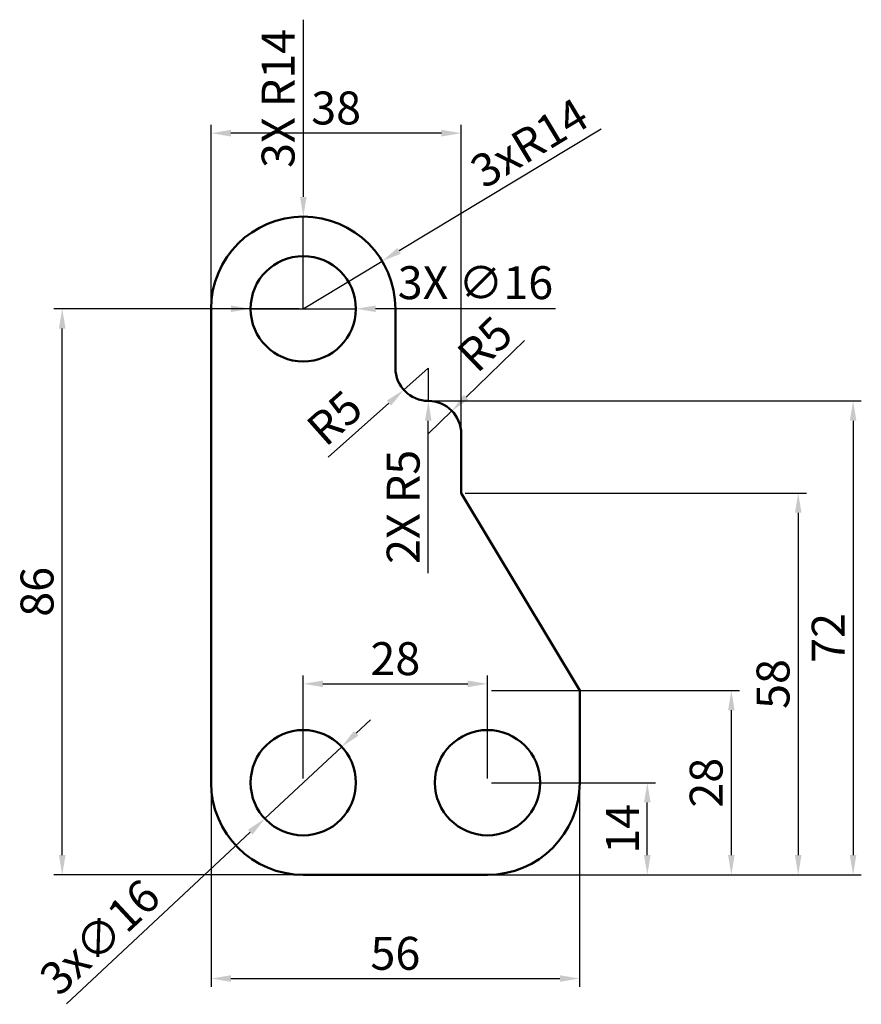
# Model space of a CAD drawing. Units: millimetres. Extents: x 41 to 168, y 30 to 180.
import ezdxf

# ---------------------------------------------------------------- set-up
doc = ezdxf.new("R2010")
doc.units = ezdxf.units.MM
doc.layers.add('M-DIMS', color=2, linetype='Continuous', lineweight=25)
doc.layers.add('M-OUTL', color=7, linetype='Continuous', lineweight=50)
doc.styles.get("Standard").update_dxf_attribs({"font": 'arial.ttf'})
doc.dimstyles.new('ISO-25', dxfattribs={"dimtxt": 5, "dimasz": 3, "dimexe": 1.25, "dimexo": 0.625, "dimtad": 1, "dimtxsty": 'Standard', "dimcen": 2.5, "dimadec": 0, "dimazin": 0, "dimtfac": 1, "dimtmove": 0, "dimatfit": 3, "dimfxl": 1, "dimarcsym": 0})

# ---------------------------------------------------------------- blocks, each defined once
blk = doc.blocks.new('*D1')
at = {"layer": 'Defpoints', "color": 0, "transparency": 16777216}
for p in [(111.68, 79.11), (83.68, 64.09), (111.68, 64.09)]:
    blk.add_point(p, dxfattribs=at)
at = {"layer": 'M-DIMS', "color": 0, "lineweight": -2, "transparency": 16777216}
for p, q in [((83.68, 64.72), (83.68, 80.36)), ((111.68, 64.72), (111.68, 80.36)), ((86.68, 79.11), (108.68, 79.11))]:
    blk.add_line(p, q, dxfattribs=at)
at = {"layer": 'M-DIMS', "color": 0, "transparency": 16777216}
for points in [[(86.68, 79.61), (86.68, 78.61), (83.68, 79.11)], [(108.68, 79.61), (108.68, 78.61), (111.68, 79.11)]]:
    blk.add_solid(points, dxfattribs=at)
at = {"layer": 'M-DIMS', "color": 0, "transparency": 16777216, "insert": (97.68, 82.29), "char_height": 5, "attachment_point": 5}
blk.add_mtext('28', dxfattribs=at)
blk = doc.blocks.new('*D2')
at = {"layer": 'Defpoints', "color": 0, "transparency": 16777216}
for p in [(111.68, 78.09), (148.73, 78.09), (111.68, 50.09)]:
    blk.add_point(p, dxfattribs=at)
at = {"layer": 'M-DIMS', "color": 0, "lineweight": -2, "transparency": 16777216}
for p, q in [((112.31, 78.09), (149.98, 78.09)), ((148.73, 53.09), (148.73, 75.09)), ((112.31, 50.09), (149.98, 50.09))]:
    blk.add_line(p, q, dxfattribs=at)
at = {"layer": 'M-DIMS', "color": 0, "transparency": 16777216}
for points in [[(148.23, 75.09), (149.23, 75.09), (148.73, 78.09)], [(148.23, 53.09), (149.23, 53.09), (148.73, 50.09)]]:
    blk.add_solid(points, dxfattribs=at)
at = {"layer": 'M-DIMS', "color": 0, "transparency": 16777216, "insert": (145.55, 64.09), "char_height": 5, "attachment_point": 5, "rotation": 90}
blk.add_mtext('28', dxfattribs=at)
blk = doc.blocks.new('*D3')
at = {"layer": 'Defpoints', "color": 0, "transparency": 16777216}
for p in [(111.68, 64.09), (135.96, 64.09), (111.68, 50.09)]:
    blk.add_point(p, dxfattribs=at)
at = {"layer": 'M-DIMS', "color": 0, "lineweight": -2, "transparency": 16777216}
for p, q in [((112.31, 64.09), (137.21, 64.09)), ((135.96, 53.09), (135.96, 61.09)), ((112.31, 50.09), (137.21, 50.09))]:
    blk.add_line(p, q, dxfattribs=at)
at = {"layer": 'M-DIMS', "color": 0, "transparency": 16777216}
for points in [[(135.46, 61.09), (136.46, 61.09), (135.96, 64.09)], [(135.46, 53.09), (136.46, 53.09), (135.96, 50.09)]]:
    blk.add_solid(points, dxfattribs=at)
at = {"layer": 'M-DIMS', "color": 0, "transparency": 16777216, "insert": (132.83, 57.09), "char_height": 5, "attachment_point": 5, "rotation": 90}
blk.add_mtext('14', dxfattribs=at)
blk = doc.blocks.new('*D4')
at = {"layer": 'Defpoints', "color": 0, "transparency": 16777216}
for p in [(102.68, 122.09), (102.68, 50.09), (167.23, 50.09)]:
    blk.add_point(p, dxfattribs=at)
at = {"layer": 'M-DIMS', "color": 0, "lineweight": -2, "transparency": 16777216}
for p, q in [((103.31, 122.09), (168.48, 122.09)), ((167.23, 119.09), (167.23, 53.09)), ((103.31, 50.09), (168.48, 50.09))]:
    blk.add_line(p, q, dxfattribs=at)
at = {"layer": 'M-DIMS', "color": 0, "transparency": 16777216}
for points in [[(166.73, 119.09), (167.73, 119.09), (167.23, 122.09)], [(166.73, 53.09), (167.73, 53.09), (167.23, 50.09)]]:
    blk.add_solid(points, dxfattribs=at)
at = {"layer": 'M-DIMS', "color": 0, "transparency": 16777216, "insert": (164.09, 86.09), "char_height": 5, "attachment_point": 5, "rotation": 90}
blk.add_mtext('72', dxfattribs=at)
blk = doc.blocks.new('*D5')
at = {"layer": 'Defpoints', "color": 0, "transparency": 16777216}
for p in [(107.68, 108.09), (107.68, 50.09), (158.89, 50.09)]:
    blk.add_point(p, dxfattribs=at)
at = {"layer": 'M-DIMS', "color": 0, "lineweight": -2, "transparency": 16777216}
for p, q in [((108.31, 108.09), (160.14, 108.09)), ((158.89, 105.09), (158.89, 53.09)), ((108.31, 50.09), (160.14, 50.09))]:
    blk.add_line(p, q, dxfattribs=at)
at = {"layer": 'M-DIMS', "color": 0, "transparency": 16777216}
for points in [[(158.39, 105.09), (159.39, 105.09), (158.89, 108.09)], [(158.39, 53.09), (159.39, 53.09), (158.89, 50.09)]]:
    blk.add_solid(points, dxfattribs=at)
at = {"layer": 'M-DIMS', "color": 0, "transparency": 16777216, "insert": (155.71, 79.09), "char_height": 5, "attachment_point": 5, "rotation": 90}
blk.add_mtext('58', dxfattribs=at)
blk = doc.blocks.new('*D6')
at = {"layer": 'Defpoints', "color": 0, "transparency": 16777216}
for p in [(69.68, 64.09), (125.68, 64.09), (125.68, 34.34)]:
    blk.add_point(p, dxfattribs=at)
at = {"layer": 'M-DIMS', "color": 0, "lineweight": -2, "transparency": 16777216}
for p, q in [((69.68, 63.47), (69.68, 33.09)), ((125.68, 63.47), (125.68, 33.09)), ((72.68, 34.34), (122.68, 34.34))]:
    blk.add_line(p, q, dxfattribs=at)
at = {"layer": 'M-DIMS', "color": 0, "transparency": 16777216}
for points in [[(72.68, 34.84), (72.68, 33.84), (69.68, 34.34)], [(122.68, 34.84), (122.68, 33.84), (125.68, 34.34)]]:
    blk.add_solid(points, dxfattribs=at)
at = {"layer": 'M-DIMS', "color": 0, "transparency": 16777216, "insert": (97.68, 37.52), "char_height": 5, "attachment_point": 5}
blk.add_mtext('56', dxfattribs=at)
blk = doc.blocks.new('*D7')
at = {"layer": 'Defpoints', "color": 0, "transparency": 16777216}
for p in [(47.06, 136.09), (83.68, 136.09), (83.68, 50.09)]:
    blk.add_point(p, dxfattribs=at)
at = {"layer": 'M-DIMS', "color": 0, "lineweight": -2, "transparency": 16777216}
for p, q in [((83.06, 136.09), (45.81, 136.09)), ((47.06, 53.09), (47.06, 133.09)), ((83.06, 50.09), (45.81, 50.09))]:
    blk.add_line(p, q, dxfattribs=at)
at = {"layer": 'M-DIMS', "color": 0, "transparency": 16777216}
for points in [[(46.56, 133.09), (47.56, 133.09), (47.06, 136.09)], [(46.56, 53.09), (47.56, 53.09), (47.06, 50.09)]]:
    blk.add_solid(points, dxfattribs=at)
at = {"layer": 'M-DIMS', "color": 0, "transparency": 16777216, "insert": (43.88, 93.09), "char_height": 5, "attachment_point": 5, "rotation": 90}
blk.add_mtext('86', dxfattribs=at)
blk = doc.blocks.new('*D8')
at = {"layer": 'Defpoints', "color": 0, "transparency": 16777216}
for p in [(69.68, 162.77), (69.68, 117.09), (107.68, 117.09)]:
    blk.add_point(p, dxfattribs=at)
at = {"layer": 'M-DIMS', "color": 0, "lineweight": -2, "transparency": 16777216}
for p, q in [((69.68, 117.72), (69.68, 164.02)), ((107.68, 117.72), (107.68, 164.02)), ((104.68, 162.77), (72.68, 162.77))]:
    blk.add_line(p, q, dxfattribs=at)
at = {"layer": 'M-DIMS', "color": 0, "transparency": 16777216}
for points in [[(72.68, 163.27), (72.68, 162.27), (69.68, 162.77)], [(104.68, 163.27), (104.68, 162.27), (107.68, 162.77)]]:
    blk.add_solid(points, dxfattribs=at)
at = {"layer": 'M-DIMS', "color": 0, "transparency": 16777216, "insert": (88.68, 165.95), "char_height": 5, "attachment_point": 5}
blk.add_mtext('38', dxfattribs=at)
blk = doc.blocks.new('*D9')
at = {"layer": 'Defpoints', "color": 0, "transparency": 16777216}
for p in [(95.67, 143.33), (83.68, 136.09)]:
    blk.add_point(p, dxfattribs=at)
at = {"layer": 'M-DIMS', "color": 0, "lineweight": -2, "transparency": 16777216}
for p, q in [((128.93, 163.4), (98.24, 144.88)), ((83.68, 136.09), (95.67, 143.33))]:
    blk.add_line(p, q, dxfattribs=at)
at = {"layer": 'M-DIMS', "color": 0, "transparency": 16777216}
blk.add_solid([(97.98, 145.31), (98.5, 144.45), (95.67, 143.33)], dxfattribs=at)
at = {"layer": 'M-DIMS', "color": 0, "transparency": 16777216, "insert": (118.37, 160.74), "char_height": 5, "attachment_point": 5, "rotation": 31.1144}
blk.add_mtext('3xR14', dxfattribs=at)
blk = doc.blocks.new('*D10')
at = {"layer": 'Defpoints', "color": 0, "transparency": 16777216}
for p in [(102.68, 127.09), (98.95, 123.77)]:
    blk.add_point(p, dxfattribs=at)
at = {"layer": 'M-DIMS', "color": 0, "lineweight": -2, "transparency": 16777216}
for p, q in [((102.68, 127.09), (98.95, 123.77)), ((87.49, 113.55), (96.71, 121.77))]:
    blk.add_line(p, q, dxfattribs=at)
at = {"layer": 'M-DIMS', "color": 0, "transparency": 16777216}
blk.add_solid([(96.38, 122.14), (97.04, 121.4), (98.95, 123.77)], dxfattribs=at)
at = {"layer": 'M-DIMS', "color": 0, "transparency": 16777216, "insert": (88.87, 119.03), "char_height": 5, "attachment_point": 5, "rotation": 41.7012}
blk.add_mtext('R5', dxfattribs=at)
blk = doc.blocks.new('*D11')
at = {"layer": 'Defpoints', "color": 0, "transparency": 16777216}
for p in [(89.53, 69.55), (77.84, 58.63)]:
    blk.add_point(p, dxfattribs=at)
at = {"layer": 'M-DIMS', "color": 0, "lineweight": -2, "transparency": 16777216}
for p, q in [((91.73, 71.6), (93.92, 73.65)), ((89.53, 69.55), (77.84, 58.63)), ((47.72, 30.52), (75.64, 56.59))]:
    blk.add_line(p, q, dxfattribs=at)
at = {"layer": 'M-DIMS', "color": 0, "transparency": 16777216}
for points in [[(91.38, 71.96), (92.07, 71.23), (89.53, 69.55)], [(75.3, 56.95), (75.99, 56.22), (77.84, 58.63)]]:
    blk.add_solid(points, dxfattribs=at)
at = {"layer": 'M-DIMS', "color": 0, "transparency": 16777216, "insert": (53.21, 40.18), "char_height": 5, "attachment_point": 5, "rotation": 43.0337}
blk.add_mtext('3x∅16', dxfattribs=at)
blk = doc.blocks.new('*D12')
at = {"layer": 'Defpoints', "color": 0, "transparency": 16777216}
for p in [(106.27, 120.57), (102.68, 117.09)]:
    blk.add_point(p, dxfattribs=at)
at = {"layer": 'M-DIMS', "color": 0, "lineweight": -2, "transparency": 16777216}
for p, q in [((117.29, 131.26), (108.43, 122.66)), ((102.68, 117.09), (106.27, 120.57))]:
    blk.add_line(p, q, dxfattribs=at)
at = {"layer": 'M-DIMS', "color": 0, "transparency": 16777216}
blk.add_solid([(108.08, 123.02), (108.78, 122.3), (106.27, 120.57)], dxfattribs=at)
at = {"layer": 'M-DIMS', "color": 0, "transparency": 16777216, "insert": (111.73, 130.28), "char_height": 5, "attachment_point": 5, "rotation": 44.1153}
blk.add_mtext('R5', dxfattribs=at)
blk = doc.blocks.new('MOUNTING-HOLE-D16')
blk.add_circle((8, 8), 8)
blk = doc.blocks.new('*D14')
at = {"layer": 'Defpoints', "color": 0, "transparency": 16777216}
for p in [(83.69, 150.09), (83.68, 136.09)]:
    blk.add_point(p, dxfattribs=at)
at = {"layer": 'M-DIMS', "color": 0, "lineweight": -2, "transparency": 16777216}
for p, q in [((83.69, 180.01), (83.69, 153.09)), ((83.68, 136.09), (83.69, 150.09))]:
    blk.add_line(p, q, dxfattribs=at)
at = {"layer": 'M-DIMS', "color": 0, "transparency": 16777216}
blk.add_solid([(83.19, 153.09), (84.19, 153.09), (83.69, 150.09)], dxfattribs=at)
at = {"layer": 'M-DIMS', "color": 0, "transparency": 16777216, "insert": (80.51, 168.05), "char_height": 5, "attachment_point": 5, "rotation": 89.9984}
blk.add_mtext('3X R14', dxfattribs=at)
blk = doc.blocks.new('*D15')
at = {"layer": 'Defpoints', "color": 0, "transparency": 16777216}
for p in [(102.68, 127.09), (102.68, 122.09)]:
    blk.add_point(p, dxfattribs=at)
at = {"layer": 'M-DIMS', "color": 0, "lineweight": -2, "transparency": 16777216}
for p, q in [((102.68, 127.09), (102.68, 122.09)), ((102.68, 95.91), (102.68, 119.09))]:
    blk.add_line(p, q, dxfattribs=at)
at = {"layer": 'M-DIMS', "color": 0, "transparency": 16777216}
blk.add_solid([(102.18, 119.09), (103.18, 119.09), (102.68, 122.09)], dxfattribs=at)
at = {"layer": 'M-DIMS', "color": 0, "transparency": 16777216, "insert": (99.51, 106), "char_height": 5, "attachment_point": 5, "rotation": 89.9998}
blk.add_mtext('2X R5', dxfattribs=at)
blk = doc.blocks.new('*D16')
at = {"layer": 'Defpoints', "color": 0, "transparency": 16777216}
for p in [(75.68, 136.09), (91.68, 136.09)]:
    blk.add_point(p, dxfattribs=at)
at = {"layer": 'M-DIMS', "color": 0, "lineweight": -2, "transparency": 16777216}
for p, q in [((72.68, 136.09), (69.68, 136.09)), ((75.68, 136.09), (91.68, 136.09)), ((122.01, 136.09), (94.68, 136.09))]:
    blk.add_line(p, q, dxfattribs=at)
at = {"layer": 'M-DIMS', "color": 0, "transparency": 16777216}
for points in [[(72.68, 136.59), (72.68, 135.59), (75.68, 136.09)], [(94.68, 136.59), (94.68, 135.59), (91.68, 136.09)]]:
    blk.add_solid(points, dxfattribs=at)
at = {"layer": 'M-DIMS', "color": 0, "transparency": 16777216, "insert": (109.85, 139.41), "char_height": 5, "attachment_point": 5, "rotation": 0.0029}
blk.add_mtext('3X ∅16', dxfattribs=at)

msp = doc.modelspace()

# ---------------------------------------------------------------- linework, layer by layer
at = {"layer": 'M-OUTL'}
for p, q in [((69.685, 64.093), (69.685, 136.093)), ((97.685, 136.093), (97.685, 127.093)), ((102.685, 122.093), (102.685, 122.093)), ((107.685, 117.093), (107.685, 108.093)), ((107.685, 108.093), (125.685, 78.093)), ((125.685, 64.093), (125.685, 78.093)), ((83.685, 50.093), (111.685, 50.093))]:
    msp.add_line(p, q, dxfattribs=at)
for centre, radius, start, end in [((83.685, 136.093), 14, 0, 180), ((102.685, 127.093), 5, 180, 270), ((102.685, 117.093), 5, 0, 90), ((83.685, 64.093), 14, 180, 270), ((111.685, 64.093), 14, 270, 0)]:
    msp.add_arc(centre, radius, start, end, dxfattribs=at)

# ---------------------------------------------------------------- block references
for p in [(75.685, 128.093), (75.685, 56.093), (103.685, 56.093)]:
    msp.add_blockref('MOUNTING-HOLE-D16', p, dxfattribs=at)

# ---------------------------------------------------------------- dimensions: what is measured, and where the dimension line sits
at = {"layer": 'M-DIMS'}
for center, mpoint, text, picture, middle in [((83.685, 136.093), (83.685, 150.093), '3X <>', '*D14', (80.506, 168.051)), ((102.685, 127.093), (102.685, 122.093), '2X <>', '*D15', (99.507, 106.003))]:
    dim = msp.add_radius_dim(center=center, mpoint=mpoint, text=text, dimstyle='ISO-25', override={"dimdec": 0, "dimlfac": 1, "dimrnd": 0, "dimzin": 0, "dimdsep": 46, "dimlunit": 2}, dxfattribs=at)
    dim.commit()
    dim.dimension.update_dxf_attribs({"geometry": picture, "text_midpoint": middle})
for base, p1, p2, picture, middle in [((69.685, 162.767), (107.685, 117.093), (69.685, 117.093), '*D8', (88.685, 165.947)), ((111.685, 79.108), (83.685, 64.093), (111.685, 64.093), '*D1', (97.685, 82.286)), ((125.685, 34.344), (69.685, 64.093), (125.685, 64.093), '*D6', (97.685, 37.522))]:
    dim = msp.add_linear_dim(base=base, p1=p1, p2=p2, dimstyle='ISO-25', override={"dimclrd": 0, "dimclre": 0, "dimclrt": 0}, dxfattribs=at)
    dim.commit()
    dim.dimension.update_dxf_attribs({"geometry": picture, "text_midpoint": middle})
dim = msp.add_radius_dim(center=(83.685, 136.093), mpoint=(95.671, 143.327), text='3x<>', dimstyle='ISO-25', override={"dimclrd": 0, "dimclre": 0, "dimclrt": 0}, dxfattribs=at)
dim.commit()
dim.dimension.update_dxf_attribs({"geometry": '*D9', "text_midpoint": (120.017, 158.022), "dimtype": 164})
dim = msp.add_diameter_dim_2p(p1=(75.685, 136.092), p2=(91.685, 136.093), text='3X <>', dimstyle='ISO-25', override={"dimdec": 0, "dimlfac": 1, "dimrnd": 0, "dimzin": 0, "dimdsep": 46, "dimlunit": 2}, dxfattribs=at)
dim.commit()
dim.dimension.update_dxf_attribs({"geometry": '*D16', "text_midpoint": (109.846, 136.094)})
for base, p1, p2, picture, middle in [((47.056, 136.093), (83.685, 50.093), (83.685, 136.093), '*D7', (43.878, 93.093)), ((167.228, 50.093), (102.685, 122.093), (102.685, 50.093), '*D4', (164.093, 86.093)), ((158.891, 50.093), (107.685, 108.093), (107.685, 50.093), '*D5', (155.713, 79.093)), ((148.726, 78.093), (111.685, 50.093), (111.685, 78.093), '*D2', (145.548, 64.093)), ((135.963, 64.093), (111.685, 50.093), (111.685, 64.093), '*D3', (132.828, 57.093))]:
    dim = msp.add_linear_dim(base=base, p1=p1, p2=p2, angle=90, dimstyle='ISO-25', override={"dimclrd": 0, "dimclre": 0, "dimclrt": 0}, dxfattribs=at)
    dim.commit()
    dim.dimension.update_dxf_attribs({"geometry": picture, "text_midpoint": middle})
for center, mpoint, picture, middle in [((102.685, 117.093), (106.274, 120.573), '*D12', (111.733, 130.278)), ((102.685, 127.093), (98.951, 123.766), '*D10', (88.874, 119.03))]:
    dim = msp.add_radius_dim(center=center, mpoint=mpoint, dimstyle='ISO-25', override={"dimclrd": 0, "dimclre": 0, "dimclrt": 0}, dxfattribs=at)
    dim.commit()
    dim.dimension.update_dxf_attribs({"geometry": picture, "text_midpoint": middle})
dim = msp.add_diameter_dim_2p(p1=(89.532, 69.552), p2=(77.837, 58.633), text='3x<>', dimstyle='ISO-25', override={"dimclrd": 0, "dimclre": 0, "dimclrt": 0}, dxfattribs=at)
dim.commit()
dim.dimension.update_dxf_attribs({"geometry": '*D11', "text_midpoint": (55.478, 37.758), "dimtype": 163})

doc.saveas('drawing.dxf')
